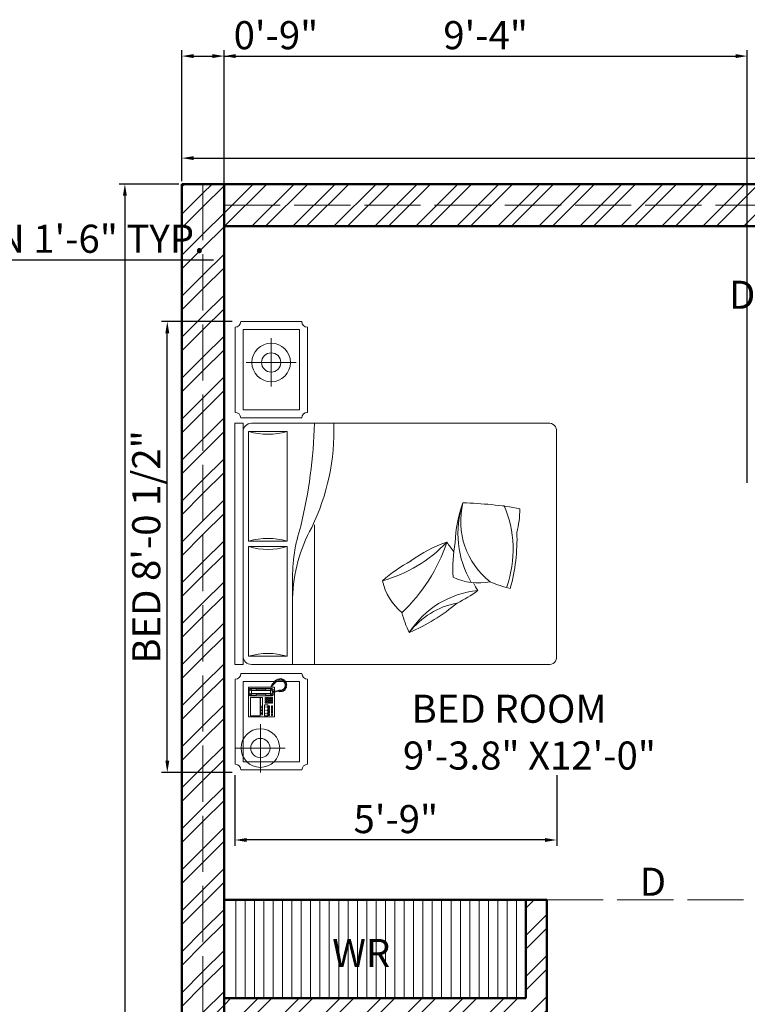
# Model space of a CAD drawing. Units: millimetres. Extents: x 4237 to 5109, y 21391 to 22486.
# Tile 16 of 17: x 4678 to 4833, y 22265 to 22476. Entities that reach past the tile are written whole.
import ezdxf

# ---------------------------------------------------------------- set-up
doc = ezdxf.new("R2010")
doc.units = ezdxf.units.MM
doc.linetypes.add('ACAD_ISO02W100', pattern=[15, 12, -3])
for name, color, linetype, lineweight in [('A-ANNO-DIMS', 2, 'Continuous', 18), ('A-ANNO-TEXT', 7, 'Continuous', 18), ('A-AREA-IDEN', 3, 'Continuous', 18), ('A-FLOR-OVHD', 1, 'ACAD_ISO02W100', 18), ('A-FURN', 8, 'Continuous', 18), ('A-FURN-CASE', 31, 'Continuous', 13), ('A-WALL', 7, 'Continuous', 50), ('A-WALL-PATT', 252, 'Continuous', 13)]:
    doc.layers.add(name, color=color, linetype=linetype, lineweight=lineweight)
doc.styles.get("Standard").update_dxf_attribs({"font": 'arial.ttf'})
doc.dimstyles.new('ISO-25', dxfattribs={"dimtxt": 6, "dimasz": 2.5, "dimexe": 1.25, "dimexo": 0.625, "dimtad": 1, "dimdec": 1, "dimlunit": 4, "dimtxsty": 'Standard', "dimcen": 2.5, "dimadec": 0, "dimazin": 0, "dimtfac": 1, "dimtdec": 1, "dimtmove": 0, "dimatfit": 3, "dimfxl": 1, "dimarcsym": 0})

# ---------------------------------------------------------------- blocks, each defined once
blk = doc.blocks.new('A$C07097A50')
for p, q in [((0.0153, 1.9631), (0.0153, 1.5831)), ((0.0503, 1.9981), (0.5803, 1.9981)), ((0.1513, 1.6872), (0.1513, 1.9968)), ((0.6153, 1.9631), (0.6153, 1.5831)), ((0.6716, 1.9489), (0.6716, 2.0001)), ((0.6716, 2.0001), (2.1719, 2.0001)), ((2.1719, 1.9489), (2.1719, 2.0001)), ((2.2051, 1.9643), (2.2051, 1.5843)), ((2.7701, 1.9993), (2.2401, 1.9993)), ((2.8051, 1.9643), (2.8051, 1.5843)), ((0.0653, 1.9481), (0.0653, 1.5981)), ((0.0653, 1.9481), (0.5653, 1.9481)), ((0.3481, 1.9163), (0.3458, 1.914)), ((0.3458, 1.914), (0.3458, 1.7563)), ((0.3481, 1.9163), (0.5287, 1.9163)), ((0.3526, 1.9037), (0.3526, 1.8431)), ((0.4669, 1.9037), (0.3526, 1.9037)), ((0.4669, 1.8431), (0.4669, 1.9037)), ((0.4772, 1.9071), (0.4818, 1.9129)), ((0.4772, 1.7688), (0.4772, 1.9071)), ((0.4818, 1.9094), (0.4807, 1.9049)), ((0.4807, 1.9049), (0.4807, 1.874)), ((0.4807, 1.9049), (0.4909, 1.8946)), ((0.4818, 1.9129), (0.5161, 1.9129)), ((0.4864, 1.9117), (0.4818, 1.9094)), ((0.4921, 1.8969), (0.4864, 1.9117)), ((0.4864, 1.9117), (0.5138, 1.9117)), ((0.5081, 1.8969), (0.5138, 1.9117)), ((0.5195, 1.9049), (0.5092, 1.8946)), ((0.5138, 1.9117), (0.5184, 1.9094)), ((0.5161, 1.9129), (0.5218, 1.9071)), ((0.5184, 1.9094), (0.5195, 1.9049)), ((0.5195, 1.9049), (0.5195, 1.874)), ((0.5218, 1.9071), (0.5218, 1.77)), ((0.5287, 1.9163), (0.5309, 1.914)), ((0.5309, 1.914), (0.5309, 1.7563)), ((0.5653, 1.9481), (0.5653, 1.5981)), ((2.1719, 1.9489), (0.6716, 1.9489)), ((2.2551, 1.9493), (2.2551, 1.5993)), ((2.7551, 1.9493), (2.2551, 1.9493)), ((2.5505, 1.6201), (2.5505, 1.9296)), ((2.7551, 1.9493), (2.7551, 1.5993)), ((0, 1.8416), (0.3001, 1.8416)), ((0.3526, 1.8431), (0.4669, 1.8431)), ((0.3572, 1.8409), (0.3572, 1.8294)), ((0.4669, 1.8409), (0.3572, 1.8409)), ((0.3664, 1.8409), (0.3664, 1.8294)), ((0.3755, 1.8409), (0.3755, 1.8294)), ((0.3846, 1.8409), (0.3846, 1.8294)), ((0.3938, 1.8409), (0.3938, 1.8294)), ((0.4029, 1.8409), (0.4029, 1.8294)), ((0.4121, 1.8409), (0.4121, 1.8294)), ((0.4669, 1.8294), (0.4669, 1.8409)), ((0.4807, 1.874), (0.4829, 1.8683)), ((0.4829, 1.8683), (0.4864, 1.8626)), ((0.4864, 1.8626), (0.4875, 1.8546)), ((0.4875, 1.8546), (0.4875, 1.8431)), ((0.4875, 1.8214), (0.4875, 1.8431)), ((0.4909, 1.8946), (0.4921, 1.8969)), ((0.4909, 1.8431), (0.4909, 1.8946)), ((0.4909, 1.8431), (0.4909, 1.7814)), ((0.5081, 1.8969), (0.4921, 1.8969)), ((0.5092, 1.8946), (0.5081, 1.8969)), ((0.5092, 1.8431), (0.5092, 1.8946)), ((0.5092, 1.8431), (0.5092, 1.7814)), ((0.5138, 1.8626), (0.5127, 1.8546)), ((0.5127, 1.8546), (0.5127, 1.8431)), ((0.5127, 1.8214), (0.5127, 1.8431)), ((0.5172, 1.8683), (0.5138, 1.8626)), ((0.5195, 1.874), (0.5172, 1.8683)), ((0.6716, 1.8977), (0.6716, 0.0512)), ((2.1719, 0.0512), (2.1719, 1.8977)), ((0.4201, 1.8168), (0.3526, 1.8168)), ((0.3526, 1.8168), (0.3526, 1.7963)), ((0.3526, 1.7963), (0.4201, 1.7963)), ((0.3652, 1.7906), (0.3538, 1.7906)), ((0.3538, 1.7906), (0.3538, 1.786)), ((0.3538, 1.786), (0.3652, 1.786)), ((0.3572, 1.8294), (0.4669, 1.8294)), ((0.3675, 1.8146), (0.3641, 1.8146)), ((0.3641, 1.8146), (0.3641, 1.8111)), ((0.3641, 1.8111), (0.3675, 1.8111)), ((0.3641, 1.802), (0.3641, 1.7986)), ((0.3675, 1.802), (0.3641, 1.802)), ((0.3641, 1.7986), (0.3675, 1.7986)), ((0.3652, 1.786), (0.3652, 1.7906)), ((0.3675, 1.8111), (0.3675, 1.8146)), ((0.3675, 1.7986), (0.3675, 1.802)), ((0.3812, 1.7906), (0.3698, 1.7906)), ((0.3698, 1.7906), (0.3698, 1.786)), ((0.3698, 1.786), (0.3812, 1.786)), ((0.3812, 1.786), (0.3812, 1.7906)), ((0.3846, 1.8146), (0.3846, 1.8111)), ((0.3881, 1.8146), (0.3846, 1.8146)), ((0.3846, 1.8111), (0.3881, 1.8111)), ((0.3846, 1.802), (0.3846, 1.7986)), ((0.3881, 1.802), (0.3846, 1.802)), ((0.3846, 1.7986), (0.3881, 1.7986)), ((0.3972, 1.7906), (0.3858, 1.7906)), ((0.3858, 1.7906), (0.3858, 1.786)), ((0.3858, 1.786), (0.3972, 1.786)), ((0.3881, 1.8111), (0.3881, 1.8146)), ((0.3881, 1.7986), (0.3881, 1.802)), ((0.3972, 1.786), (0.3972, 1.7906)), ((0.4018, 1.7906), (0.4018, 1.786)), ((0.4132, 1.7906), (0.4018, 1.7906)), ((0.4018, 1.786), (0.4132, 1.786)), ((0.4052, 1.8146), (0.4052, 1.8111)), ((0.4086, 1.8146), (0.4052, 1.8146)), ((0.4052, 1.8111), (0.4086, 1.8111)), ((0.4052, 1.802), (0.4052, 1.7986)), ((0.4086, 1.802), (0.4052, 1.802)), ((0.4052, 1.7986), (0.4086, 1.7986)), ((0.4086, 1.8111), (0.4086, 1.8146)), ((0.4086, 1.7986), (0.4086, 1.802)), ((0.4132, 1.786), (0.4132, 1.7906)), ((0.4201, 1.7963), (0.4201, 1.8168)), ((0.4304, 1.8111), (0.4395, 1.8111)), ((0.4304, 1.8043), (0.4304, 1.8111)), ((0.4395, 1.8043), (0.4304, 1.8043)), ((0.4304, 1.7986), (0.4395, 1.7986)), ((0.4304, 1.7917), (0.4304, 1.7986)), ((0.4395, 1.7917), (0.4304, 1.7917)), ((0.4304, 1.778), (0.4304, 1.7848)), ((0.4304, 1.7848), (0.4395, 1.7848)), ((0.4395, 1.778), (0.4304, 1.778)), ((0.4395, 1.8111), (0.4395, 1.8043)), ((0.4395, 1.7986), (0.4395, 1.7917)), ((0.4395, 1.7848), (0.4395, 1.778)), ((0.4441, 1.8043), (0.4441, 1.8111)), ((0.4441, 1.8111), (0.4532, 1.8111)), ((0.4532, 1.8043), (0.4441, 1.8043)), ((0.4441, 1.7986), (0.4532, 1.7986)), ((0.4441, 1.7917), (0.4441, 1.7986)), ((0.4532, 1.7917), (0.4441, 1.7917)), ((0.4441, 1.778), (0.4441, 1.7848)), ((0.4441, 1.7848), (0.4532, 1.7848)), ((0.4532, 1.778), (0.4441, 1.778)), ((0.4532, 1.8111), (0.4532, 1.8043)), ((0.4532, 1.7986), (0.4532, 1.7917)), ((0.4532, 1.7848), (0.4532, 1.778)), ((0.4578, 1.8111), (0.4669, 1.8111)), ((0.4578, 1.8043), (0.4578, 1.8111)), ((0.4669, 1.8043), (0.4578, 1.8043)), ((0.4578, 1.7986), (0.4669, 1.7986)), ((0.4578, 1.7917), (0.4578, 1.7986)), ((0.4669, 1.7917), (0.4578, 1.7917)), ((0.4578, 1.7791), (0.4578, 1.786)), ((0.4578, 1.786), (0.4669, 1.786)), ((0.4669, 1.7791), (0.4578, 1.7791)), ((0.4669, 1.8111), (0.4669, 1.8043)), ((0.4669, 1.7986), (0.4669, 1.7917)), ((0.4669, 1.786), (0.4669, 1.7791)), ((0.4807, 1.802), (0.4829, 1.8077)), ((0.4807, 1.7711), (0.4807, 1.802)), ((0.4807, 1.7711), (0.4909, 1.7814)), ((0.4829, 1.8077), (0.4864, 1.8134)), ((0.4864, 1.8134), (0.4875, 1.8214)), ((0.4921, 1.7791), (0.4864, 1.7643)), ((0.4909, 1.7814), (0.4921, 1.7791)), ((0.5081, 1.7791), (0.4921, 1.7791)), ((0.5092, 1.7814), (0.5081, 1.7791)), ((0.5081, 1.7791), (0.5138, 1.7643)), ((0.5195, 1.7711), (0.5092, 1.7814)), ((0.5138, 1.8134), (0.5127, 1.8214)), ((0.5172, 1.8077), (0.5138, 1.8134)), ((0.5195, 1.802), (0.5172, 1.8077)), ((0.5195, 1.7711), (0.5195, 1.802)), ((0.5378, 1.7743), (0.5309, 1.7768)), ((0.3458, 1.7563), (0.3481, 1.754)), ((0.5, 1.754), (0.3481, 1.754)), ((0.3538, 1.7666), (0.3538, 1.7734)), ((0.3538, 1.7734), (0.3652, 1.7734)), ((0.3652, 1.7666), (0.3538, 1.7666)), ((0.3652, 1.7734), (0.3652, 1.7666)), ((0.3698, 1.7666), (0.3698, 1.7734)), ((0.3698, 1.7734), (0.3812, 1.7734)), ((0.3812, 1.7666), (0.3698, 1.7666)), ((0.3812, 1.7734), (0.3812, 1.7666)), ((0.3858, 1.7666), (0.3858, 1.7734)), ((0.3858, 1.7734), (0.3972, 1.7734)), ((0.3972, 1.7666), (0.3858, 1.7666)), ((0.3972, 1.7734), (0.3972, 1.7666)), ((0.4018, 1.7734), (0.4132, 1.7734)), ((0.4018, 1.7666), (0.4018, 1.7734)), ((0.4132, 1.7666), (0.4018, 1.7666)), ((0.4132, 1.7734), (0.4132, 1.7666)), ((0.4304, 1.7723), (0.4395, 1.7723)), ((0.4304, 1.7654), (0.4304, 1.7723)), ((0.4395, 1.7654), (0.4304, 1.7654)), ((0.4395, 1.7723), (0.4395, 1.7654)), ((0.4441, 1.7723), (0.4532, 1.7723)), ((0.4441, 1.7654), (0.4441, 1.7723)), ((0.4532, 1.7654), (0.4441, 1.7654)), ((0.4532, 1.7723), (0.4532, 1.7654)), ((0.4578, 1.7654), (0.4578, 1.7723)), ((0.4578, 1.7723), (0.4669, 1.7723)), ((0.4669, 1.7654), (0.4578, 1.7654)), ((0.4669, 1.7723), (0.4669, 1.7654)), ((0.4829, 1.7631), (0.4772, 1.7688)), ((0.4818, 1.7666), (0.4807, 1.7711)), ((0.4864, 1.7643), (0.4818, 1.7666)), ((0.499, 1.7631), (0.4829, 1.7631)), ((0.4864, 1.7643), (0.499, 1.7643)), ((0.5024, 1.7677), (0.4989, 1.7677)), ((0.4989, 1.7677), (0.4991, 1.7578)), ((0.4991, 1.7578), (0.5019, 1.7463)), ((0.5019, 1.7463), (0.5047, 1.7354)), ((0.5026, 1.7254), (0.5021, 1.7199)), ((0.5021, 1.7199), (0.5088, 1.7187)), ((0.5088, 1.7187), (0.5023, 1.7148)), ((0.503, 1.7585), (0.5024, 1.7677)), ((0.5026, 1.7643), (0.5138, 1.7643)), ((0.5051, 1.728), (0.5026, 1.7254)), ((0.5161, 1.7631), (0.5027, 1.7631)), ((0.5047, 1.7511), (0.503, 1.7585)), ((0.5287, 1.754), (0.504, 1.754)), ((0.5047, 1.7354), (0.5044, 1.7294)), ((0.5044, 1.7294), (0.5051, 1.728)), ((0.5074, 1.7403), (0.5047, 1.7511)), ((0.5081, 1.7347), (0.5074, 1.7403)), ((0.5079, 1.7287), (0.5081, 1.7347)), ((0.5121, 1.7257), (0.5079, 1.7287)), ((0.5111, 1.7203), (0.5121, 1.7257)), ((0.5123, 1.7058), (0.5111, 1.7203)), ((0.5138, 1.7643), (0.5184, 1.7666)), ((0.5218, 1.77), (0.5161, 1.7631)), ((0.5184, 1.7666), (0.5195, 1.7711)), ((0.5309, 1.7563), (0.5287, 1.754)), ((0.5309, 1.7723), (0.536, 1.7709)), ((0.536, 1.7709), (0.5406, 1.7672)), ((0.541, 1.7711), (0.5378, 1.7743)), ((0.5406, 1.7672), (0.5418, 1.7656)), ((0.5434, 1.7689), (0.541, 1.7711)), ((0.5442, 1.7658), (0.5418, 1.7634)), ((0.5418, 1.7656), (0.5442, 1.7658)), ((0.5418, 1.7634), (0.5511, 1.7552)), ((0.5477, 1.7705), (0.5434, 1.7689)), ((0.5497, 1.7685), (0.5477, 1.7705)), ((0.5481, 1.765), (0.5497, 1.7685)), ((0.5509, 1.7672), (0.5481, 1.765)), ((0.5539, 1.764), (0.5509, 1.7672)), ((0.5511, 1.7552), (0.5662, 1.7423)), ((0.5515, 1.7574), (0.5539, 1.764)), ((0.5577, 1.7606), (0.5515, 1.7574)), ((0.563, 1.7556), (0.5577, 1.7606)), ((0.5618, 1.7483), (0.563, 1.7556)), ((0.567, 1.7515), (0.5618, 1.7483)), ((0.5664, 1.7419), (0.574, 1.7201)), ((0.5714, 1.7469), (0.567, 1.7515)), ((0.5696, 1.7419), (0.5714, 1.7469)), ((0.5766, 1.7426), (0.5697, 1.7419)), ((0.574, 1.7201), (0.5708, 1.7028)), ((0.572, 1.7331), (0.5787, 1.7356)), ((0.5794, 1.7333), (0.572, 1.7331)), ((0.5761, 1.7234), (0.581, 1.728)), ((0.5824, 1.7234), (0.5761, 1.7234)), ((0.5764, 1.7155), (0.5835, 1.7176)), ((0.5824, 1.712), (0.5764, 1.7155)), ((0.5787, 1.7356), (0.5766, 1.7426)), ((0.581, 1.728), (0.5794, 1.7333)), ((0.5835, 1.7176), (0.5824, 1.7234)), ((2.7018, 1.7745), (2.4017, 1.7745)), ((0.5023, 1.7148), (0.5028, 1.7085)), ((0.5028, 1.7085), (0.5102, 1.7078)), ((0.5102, 1.7078), (0.5037, 1.7028)), ((0.5037, 1.7028), (0.5067, 1.6974)), ((0.5067, 1.6974), (0.5137, 1.6988)), ((0.5137, 1.6988), (0.5104, 1.6923)), ((0.5104, 1.6923), (0.5139, 1.6882)), ((0.5211, 1.6947), (0.5123, 1.7058)), ((0.5139, 1.6882), (0.5192, 1.6921)), ((0.5192, 1.6921), (0.5183, 1.6859)), ((0.5183, 1.6859), (0.5227, 1.6831)), ((0.5333, 1.6882), (0.5211, 1.6947)), ((0.5227, 1.6831), (0.5282, 1.6877)), ((0.5282, 1.6877), (0.5276, 1.6801)), ((0.5276, 1.6801), (0.5324, 1.6787)), ((0.5324, 1.6787), (0.5354, 1.6849)), ((0.5472, 1.687), (0.5333, 1.6882)), ((0.5354, 1.6849), (0.5382, 1.6787)), ((0.5382, 1.6787), (0.5421, 1.6782)), ((0.5421, 1.6782), (0.5437, 1.6849)), ((0.5437, 1.6849), (0.5463, 1.6775)), ((0.5463, 1.6775), (0.5507, 1.6787)), ((0.5606, 1.6928), (0.5472, 1.687)), ((0.5507, 1.6787), (0.5509, 1.6849)), ((0.5509, 1.6849), (0.5562, 1.6803)), ((0.5562, 1.6803), (0.5599, 1.6822)), ((0.5592, 1.6891), (0.5641, 1.6831)), ((0.5599, 1.6822), (0.5592, 1.6891)), ((0.5708, 1.7028), (0.5606, 1.6928)), ((0.5641, 1.6831), (0.5678, 1.6863)), ((0.565, 1.6926), (0.5715, 1.6898)), ((0.5678, 1.6863), (0.565, 1.6926)), ((0.5745, 1.6926), (0.5713, 1.6988)), ((0.5713, 1.6988), (0.578, 1.6967)), ((0.5715, 1.6898), (0.5745, 1.6926)), ((0.5743, 1.7076), (0.5814, 1.7074)), ((0.5798, 1.7014), (0.5743, 1.7076)), ((0.578, 1.6967), (0.5798, 1.7014)), ((0.5814, 1.7074), (0.5824, 1.712)), ((0.0653, 1.5981), (0.5653, 1.5981)), ((2.7551, 1.5993), (2.2551, 1.5993)), ((0.0503, 1.5481), (0.5803, 1.5481)), ((2.7701, 1.5493), (2.2401, 1.5493)), ((0.7228, 0.0001), (2.1207, 0.0001))]:
    blk.add_line(p, q)
at = {"linetype": 'ByBlock'}
for p, q in [((0.7228, 1.6759), (0.7228, 1.9148)), ((0.7228, 1.9148), (1.4047, 1.9148)), ((1.4047, 1.9148), (1.4047, 1.6759)), ((1.4388, 1.6759), (1.4388, 1.9148)), ((1.4388, 1.9148), (2.1207, 1.9148)), ((2.1207, 1.9148), (2.1207, 1.6759)), ((1.4047, 1.6759), (0.7228, 1.6759)), ((2.1207, 1.6759), (1.4388, 1.6759)), ((1.1914, 1.6418), (0.6716, 1.6418)), ((1.5412, 1.5053), (0.6716, 1.5053))]:
    blk.add_line(p, q, dxfattribs=at)
for centre in [(0.1513, 1.8416), (2.5505, 1.7745)]:
    blk.add_circle(centre, 0.12, dxfattribs=at)
for centre in [(0.1513, 1.8416), (2.5505, 1.7745)]:
    blk.add_circle(centre, 0.06)
for centre, radius, start, end in [((0.0153, 1.9981), 0.035, 270, 0), ((0.6153, 1.9981), 0.035, 180, 270), ((2.2051, 1.9993), 0.035, 270, 0), ((2.8051, 1.9993), 0.035, 180, 270), ((0.7228, 1.8977), 0.0512, 90, 180), ((2.1207, 1.8977), 0.0512, 0, 90), ((0.0153, 1.5481), 0.035, 0, 90), ((0.6153, 1.5481), 0.035, 90, 180), ((2.2051, 1.5493), 0.035, 0, 90), ((2.8051, 1.5493), 0.035, 90, 180), ((1.2698, 0.7333), 0.3575, 102.47819, 140.46254), ((0.4476, 0.4335), 0.9879, 28.49711, 41.05657), ((2.0313, 1.3124), 0.8697, 195.33601, 226.41927), ((1.1192, 0.4274), 0.548, 103.20343, 117.03623), ((1.7756, 1.7059), 1.0798, 223.63057, 251.4288), ((1.9422, 1.372), 1.1652, 203.06416, 220.32086), ((0.5744, 0.5274), 0.4879, 10.69865, 52.68638), ((0.5678, 0.4375), 0.5655, 5.33912, 57.68949), ((0.6844, 0.4345), 0.7874, 18.35266, 36.68512), ((0.1017, 2.4319), 2.1977, 305.29657, 307.24182), ((1.7177, 0.9312), 0.734, 205.25901, 216.93514), ((1.5362, 0.487), 0.3575, 154.0418, 192.02615), ((1.4868, 0.0041), 0.6085, 71.81005, 120.13512), ((1.2599, -0.3434), 0.9879, 80.06073, 92.62018), ((1.4063, -0.1573), 0.7874, 69.91627, 88.24873), ((1.5627, 0.1186), 0.4774, 76.18494, 142.00166), ((-0.5205, 0.628), 2.1977, 349.48843, 358.80544), ((0.1017, 2.4319), 2.1977, 297.92482, 299.3793), ((1.6822, 0.1789), 0.548, 154.76704, 168.59984), ((1.3874, 0.9578), 0.6885, 250.29361, 293.6414), ((1.4539, 1.4107), 1.1652, 254.62778, 271.88448), ((1.6595, 0.9609), 0.734, 256.82263, 268.49876), ((0.717, 0.0455), 0.0458, 172.75992, 277.24008), ((2.1265, 0.0455), 0.0458, 262.75992, 7.24008)]:
    blk.add_arc(centre, radius, start, end)
for centre, radius, start, end in [((0.3133, 1.7953), 0.4265, 343.73979, 16.26021), ((1.8141, 1.7953), 0.4265, 163.73979, 196.26021), ((1.0294, 1.7953), 0.4265, 343.73979, 16.26021), ((2.5302, 1.7953), 0.4265, 163.73979, 196.26021), ((1.053, 0.6571), 0.9853, 61.43285, 88.12613), ((1.2053, 0.5713), 1.0706, 72.19663, 90.74184), ((2.2595, 4.5996), 3.0955, 256.42012, 268.37887), ((2.1283, 2.7745), 1.3903, 244.24266, 271.79845)]:
    blk.add_arc(centre, radius, start, end, dxfattribs=at)
blk = doc.blocks.new('*D59')
at = {"layer": 'A-ANNO-DIMS', "color": 0, "lineweight": -2, "transparency": 16777216}
for p, q in [((4712.61, 22441.33), (4712.61, 22447.5)), ((4715.11, 22446.25), (5070.01, 22446.25)), ((5072.51, 22436.83), (5072.51, 22447.5))]:
    blk.add_line(p, q, dxfattribs=at)
at = {"layer": 'A-ANNO-DIMS', "color": 0, "transparency": 16777216}
for points in [[(4715.11, 22446.66), (4715.11, 22445.83), (4712.61, 22446.25)], [(5070.01, 22446.66), (5070.01, 22445.83), (5072.51, 22446.25)]]:
    blk.add_solid(points, dxfattribs=at)
at = {"layer": 'Defpoints', "color": 0, "transparency": 16777216}
for p in [(5072.51, 22446.25), (4712.61, 22440.7), (5072.51, 22436.2)]:
    blk.add_point(p, dxfattribs=at)
at = {"layer": 'A-ANNO-DIMS', "color": 0, "transparency": 16777216, "insert": (4892.56, 22451.47), "char_height": 9, "attachment_point": 5}
blk.add_mtext("30'", dxfattribs=at)
blk = doc.blocks.new('*D60')
at = {"layer": 'A-ANNO-DIMS', "color": 0, "lineweight": -2, "transparency": 16777216}
for p, q in [((4711.99, 22440.7), (4699.18, 22440.7)), ((4700.43, 22438.2), (4700.43, 22018.7)), ((4711.99, 22016.2), (4699.18, 22016.2))]:
    blk.add_line(p, q, dxfattribs=at)
at = {"layer": 'A-ANNO-DIMS', "color": 0, "transparency": 16777216}
for points in [[(4700.01, 22438.2), (4700.85, 22438.2), (4700.43, 22440.7)], [(4700.01, 22018.7), (4700.85, 22018.7), (4700.43, 22016.2)]]:
    blk.add_solid(points, dxfattribs=at)
at = {"layer": 'Defpoints', "color": 0, "transparency": 16777216}
for p in [(4712.61, 22440.7), (4700.43, 22016.2), (4712.61, 22016.2)]:
    blk.add_point(p, dxfattribs=at)
at = {"layer": 'A-ANNO-DIMS', "color": 0, "transparency": 16777216, "insert": (4689.19, 22228.45), "char_height": 9, "attachment_point": 5, "rotation": 90}
blk.add_mtext('35\'-4{\\H1x;\\S1/2;}"', dxfattribs=at)
blk = doc.blocks.new('*D68')
at = {"layer": 'A-ANNO-DIMS', "color": 0, "lineweight": -2, "transparency": 16777216}
for p, q in [((4723.32, 22411.32), (4708.24, 22411.32)), ((4709.49, 22317.47), (4709.49, 22408.82)), ((4723.32, 22314.97), (4708.24, 22314.97))]:
    blk.add_line(p, q, dxfattribs=at)
at = {"layer": 'A-ANNO-DIMS', "color": 0, "transparency": 16777216}
for points in [[(4709.08, 22408.82), (4709.91, 22408.82), (4709.49, 22411.32)], [(4709.08, 22317.47), (4709.91, 22317.47), (4709.49, 22314.97)]]:
    blk.add_solid(points, dxfattribs=at)
at = {"layer": 'Defpoints', "color": 0, "transparency": 16777216}
for p in [(4709.49, 22411.32), (4723.95, 22411.32), (4723.95, 22314.97)]:
    blk.add_point(p, dxfattribs=at)
at = {"layer": 'A-ANNO-DIMS', "color": 0, "transparency": 16777216, "insert": (4705.77, 22363.15), "char_height": 6, "attachment_point": 5, "rotation": 90}
blk.add_mtext('BED 8\'-0 1/2"', dxfattribs=at)
blk = doc.blocks.new('*D69')
at = {"layer": 'A-ANNO-DIMS', "color": 0, "lineweight": -2, "transparency": 16777216}
for p, q in [((4723.95, 22314.34), (4723.95, 22299.27)), ((4792.7, 22314.34), (4792.7, 22299.27)), ((4790.2, 22300.52), (4726.45, 22300.52))]:
    blk.add_line(p, q, dxfattribs=at)
at = {"layer": 'A-ANNO-DIMS', "color": 0, "transparency": 16777216}
for points in [[(4726.45, 22300.93), (4726.45, 22300.1), (4723.95, 22300.52)], [(4790.2, 22300.93), (4790.2, 22300.1), (4792.7, 22300.52)]]:
    blk.add_solid(points, dxfattribs=at)
at = {"layer": 'Defpoints', "color": 0, "transparency": 16777216}
for p in [(4723.95, 22314.97), (4792.7, 22314.97), (4723.95, 22300.52)]:
    blk.add_point(p, dxfattribs=at)
at = {"layer": 'A-ANNO-DIMS', "color": 0, "transparency": 16777216, "insert": (4758.32, 22304.21), "char_height": 6, "attachment_point": 5}
blk.add_mtext('5\'-9"', dxfattribs=at)
blk = doc.blocks.new('*D78')
at = {"layer": 'A-ANNO-DIMS', "color": 0, "lineweight": -2, "transparency": 16777216}
for p, q in [((4622.45, 22426.58), (4622.45, 22423.25)), ((4640.45, 22426.58), (4640.45, 22423.25)), ((4624.95, 22424.5), (4637.95, 22424.5)), ((4640.45, 22424.5), (4719.36, 22424.5))]:
    blk.add_line(p, q, dxfattribs=at)
at = {"layer": 'A-ANNO-DIMS', "color": 0, "transparency": 16777216}
for points in [[(4624.95, 22424.92), (4624.95, 22424.08), (4622.45, 22424.5)], [(4637.95, 22424.92), (4637.95, 22424.08), (4640.45, 22424.5)]]:
    blk.add_solid(points, dxfattribs=at)
at = {"layer": 'Defpoints', "color": 0, "transparency": 16777216}
for p in [(4622.45, 22427.2), (4640.45, 22427.2), (4640.45, 22424.5)]:
    blk.add_point(p, dxfattribs=at)
at = {"layer": 'A-ANNO-DIMS', "color": 0, "transparency": 16777216, "insert": (4681.15, 22428.23), "char_height": 6, "attachment_point": 5}
blk.add_mtext('COLUMN 1\'-6" TYP.', dxfattribs=at)
blk = doc.blocks.new('*D112')
at = {"layer": 'A-ANNO-DIMS', "color": 0, "lineweight": -2, "transparency": 16777216}
for p, q in [((4712.61, 22441.33), (4712.61, 22469.3)), ((4721.61, 22432.33), (4721.61, 22469.3)), ((4715.11, 22468.05), (4719.11, 22468.05)), ((4721.61, 22468.05), (4741.31, 22468.05))]:
    blk.add_line(p, q, dxfattribs=at)
at = {"layer": 'A-ANNO-DIMS', "color": 0, "transparency": 16777216}
for points in [[(4715.11, 22468.47), (4715.11, 22467.63), (4712.61, 22468.05)], [(4719.11, 22468.47), (4719.11, 22467.63), (4721.61, 22468.05)]]:
    blk.add_solid(points, dxfattribs=at)
at = {"layer": 'Defpoints', "color": 0, "transparency": 16777216}
for p in [(4721.61, 22468.05), (4712.61, 22440.7), (4721.61, 22431.7)]:
    blk.add_point(p, dxfattribs=at)
at = {"layer": 'A-ANNO-DIMS', "color": 0, "transparency": 16777216, "insert": (4732.71, 22471.74), "char_height": 6, "attachment_point": 5}
blk.add_mtext('0\'-9"', dxfattribs=at)
blk = doc.blocks.new('*D113')
at = {"layer": 'A-ANNO-DIMS', "color": 0, "lineweight": -2, "transparency": 16777216}
for p, q in [((4721.61, 22432.33), (4721.61, 22469.3)), ((4833.41, 22376.83), (4833.41, 22469.3)), ((4724.11, 22468.05), (4830.91, 22468.05))]:
    blk.add_line(p, q, dxfattribs=at)
at = {"layer": 'A-ANNO-DIMS', "color": 0, "transparency": 16777216}
for points in [[(4724.11, 22468.47), (4724.11, 22467.63), (4721.61, 22468.05)], [(4830.91, 22468.47), (4830.91, 22467.63), (4833.41, 22468.05)]]:
    blk.add_solid(points, dxfattribs=at)
at = {"layer": 'Defpoints', "color": 0, "transparency": 16777216}
for p in [(4833.41, 22468.05), (4721.61, 22431.7), (4833.41, 22376.2)]:
    blk.add_point(p, dxfattribs=at)
at = {"layer": 'A-ANNO-DIMS', "color": 0, "transparency": 16777216, "insert": (4777.51, 22471.74), "char_height": 6, "attachment_point": 5}
blk.add_mtext('9\'-4"', dxfattribs=at)

msp = doc.modelspace()

# ---------------------------------------------------------------- hatches: boundary and pattern name
at = {"layer": 'A-WALL-PATT'}
h = msp.add_hatch(dxfattribs=at)
h.set_pattern_fill('ANSI32', color=256, scale=0.65)
h.paths.add_polyline_path([(4717.11, 22440.7), (4712.61, 22440.7), (4712.61, 22016.2), (4717.11, 22016.2), (4717.11, 22028.2)])
h = msp.add_hatch(dxfattribs=at)
h.set_pattern_fill('ANSI32', color=256, scale=0.65)
h.paths.add_polyline_path([(4721.61, 22440.7), (4717.11, 22440.7), (4717.11, 22028.2), (4721.61, 22028.2)])
h = msp.add_hatch(dxfattribs=at)
h.set_pattern_fill('ANSI32', color=256, scale=0.65)
h.paths.add_polyline_path([(4837.91, 22440.7), (4721.61, 22440.7), (4721.61, 22431.7), (4837.91, 22431.7)])
h = msp.add_hatch(dxfattribs=at)
h.set_pattern_fill('ANSI32', color=256, scale=0.65)
h.paths.add_polyline_path([(4790.61, 22287.7), (4786.11, 22287.7), (4786.11, 22266.7), (4721.61, 22266.7), (4721.61, 22262.2), (4786.11, 22262.2), (4786.11, 22215.7), (4790.61, 22215.7)])

# ---------------------------------------------------------------- linework, layer by layer
at = {"layer": 'A-FLOR-OVHD'}
for p, q in [((4717.11, 22440.7), (4717.11, 21972.7)), ((4721.61, 22436.2), (4915.91, 22436.2)), ((4790.61, 22287.7), (4833.41, 22287.7))]:
    msp.add_line(p, q, dxfattribs=at)
at = {"layer": 'A-FURN-CASE'}
for p, q in [((4724.11, 22287.7), (4724.11, 22266.7)), ((4726.11, 22287.7), (4726.11, 22266.7)), ((4728.11, 22287.7), (4728.11, 22266.7)), ((4730.11, 22287.7), (4730.11, 22266.7)), ((4732.11, 22287.7), (4732.11, 22266.7)), ((4734.11, 22287.7), (4734.11, 22266.7)), ((4736.11, 22287.7), (4736.11, 22266.7)), ((4738.11, 22287.7), (4738.11, 22266.7)), ((4740.11, 22287.7), (4740.11, 22266.7)), ((4742.11, 22287.7), (4742.11, 22266.7)), ((4744.11, 22287.7), (4744.11, 22266.7)), ((4746.11, 22287.7), (4746.11, 22266.7)), ((4748.11, 22287.7), (4748.11, 22266.7)), ((4750.11, 22287.7), (4750.11, 22266.7)), ((4752.11, 22287.7), (4752.11, 22266.7)), ((4754.11, 22287.7), (4754.11, 22266.7)), ((4756.11, 22287.7), (4756.11, 22266.7)), ((4758.11, 22287.7), (4758.11, 22266.7)), ((4760.11, 22287.7), (4760.11, 22266.7)), ((4762.11, 22287.7), (4762.11, 22266.7)), ((4764.11, 22287.7), (4764.11, 22266.7)), ((4766.11, 22287.7), (4766.11, 22266.7)), ((4768.11, 22287.7), (4768.11, 22266.7)), ((4770.11, 22287.7), (4770.11, 22266.7)), ((4772.11, 22287.7), (4772.11, 22266.7)), ((4774.11, 22287.7), (4774.11, 22266.7)), ((4776.11, 22287.7), (4776.11, 22266.7)), ((4778.11, 22287.7), (4778.11, 22266.7)), ((4780.11, 22287.7), (4780.11, 22266.7)), ((4782.11, 22287.7), (4782.11, 22266.7)), ((4784.11, 22287.7), (4784.11, 22266.7))]:
    msp.add_line(p, q, dxfattribs=at)
at = {"layer": 'A-WALL'}
for p, q in [((4712.61, 22440.7), (4712.61, 22016.2)), ((4712.61, 22440.7), (4837.91, 22440.7)), ((4721.61, 22440.7), (4721.61, 22028.2)), ((4721.61, 22431.7), (5054.51, 22431.7)), ((4721.61, 22287.7), (4790.61, 22287.7)), ((4786.11, 22287.7), (4786.11, 22266.7)), ((4790.61, 22287.7), (4790.61, 22215.7)), ((4721.61, 22266.7), (4786.11, 22266.7))]:
    msp.add_line(p, q, dxfattribs=at)

# ---------------------------------------------------------------- block references
at = {"layer": 'A-FURN', "xscale": 34.34793554477467, "yscale": 34.34793554477467, "zscale": 34.34793554477467, "rotation": 90}
msp.add_blockref('A$C07097A50', (4792.64, 22314.97), dxfattribs=at)

# ---------------------------------------------------------------- texts
at = {"layer": 'A-ANNO-TEXT', "char_height": 6, "attachment_point": 1}
for s, insert in [('    D', (4822.17, 22420.04)), ('    D', (4803.1, 22294.6)), ('   WR', (4739.23, 22279.36))]:
    msp.add_mtext_dynamic_manual_height_columns(s, width=21.7253, gutter_width=12.5, heights=[0], dxfattribs=dict(at, insert=insert))
at = {"layer": 'A-AREA-IDEN', "insert": (4759.85, 22331.57), "char_height": 6, "attachment_point": 1}
msp.add_mtext_dynamic_manual_height_columns(' BED ROOM \\P9\'-3.8" X12\'-0"', width=55.7646, gutter_width=12.5, heights=[0], dxfattribs=at)

# ---------------------------------------------------------------- dimensions: what is measured, and where the dimension line sits
at = {"layer": 'A-ANNO-DIMS'}
for base, p1, p2, override, picture, middle in [((4721.61, 22468.05), (4712.61, 22440.7), (4721.61, 22431.7), {"dimdec": 1, "dimlfac": 1, "dimrnd": 0, "dimzin": 1, "dimdsep": 46, "dimlunit": 4, "dimfrac": 2}, '*D112', (4732.71, 22471.74)), ((4833.41, 22468.05), (4721.61, 22431.7), (4833.41, 22376.2), {"dimdec": 1, "dimlfac": 1, "dimrnd": 0, "dimzin": 1, "dimdsep": 46, "dimlunit": 4, "dimfrac": 2}, '*D113', (4777.51, 22471.74)), ((5072.51, 22446.25), (4712.61, 22440.7), (5072.51, 22436.2), {"dimtxt": 9, "dimclrd": 0, "dimclre": 0, "dimclrt": 0}, '*D59', (4892.56, 22451.47))]:
    dim = msp.add_linear_dim(base=base, p1=p1, p2=p2, dimstyle='ISO-25', override=override, dxfattribs=at)
    dim.commit()
    dim.dimension.update_dxf_attribs({"geometry": picture, "text_midpoint": middle})
dim = msp.add_linear_dim(base=(4640.45, 22424.5), p1=(4622.45, 22427.2), p2=(4640.45, 22427.2), text='COLUMN <> TYP.', dimstyle='ISO-25', override={"dimdec": 1, "dimrnd": 0, "dimzin": 1, "dimlunit": 4, "dimfrac": 2}, dxfattribs=at)
dim.commit()
dim.dimension.update_dxf_attribs({"geometry": '*D78', "text_midpoint": (4681.15, 22428.23)})
for base, p1, p2, angle, override, picture, middle in [((4700.43, 22016.2), (4712.61, 22440.7), (4712.61, 22016.2), 90, {"dimtxt": 9, "dimclrd": 0, "dimclre": 0, "dimclrt": 0}, '*D60', (4689.19, 22228.45)), ((4723.9464, 22300.5171), (4792.7036, 22314.9697), (4723.9464, 22314.9697), 180, {"dimdec": 1, "dimrnd": 0, "dimzin": 1, "dimlunit": 4, "dimfrac": 2}, '*D69', (4758.325, 22304.2055))]:
    dim = msp.add_linear_dim(base=base, p1=p1, p2=p2, angle=angle, dimstyle='ISO-25', override=override, dxfattribs=at)
    dim.commit()
    dim.dimension.update_dxf_attribs({"geometry": picture, "text_midpoint": middle})
dim = msp.add_linear_dim(base=(4709.4937, 22411.3208), p1=(4723.9464, 22314.9697), p2=(4723.9464, 22411.3208), angle=90, text='BED <>', dimstyle='ISO-25', override={"dimdec": 1, "dimrnd": 0, "dimzin": 1, "dimlunit": 4, "dimfrac": 2}, dxfattribs=at)
dim.commit()
dim.dimension.update_dxf_attribs({"geometry": '*D68', "text_midpoint": (4705.7664, 22363.1453)})

doc.saveas('drawing.dxf')
